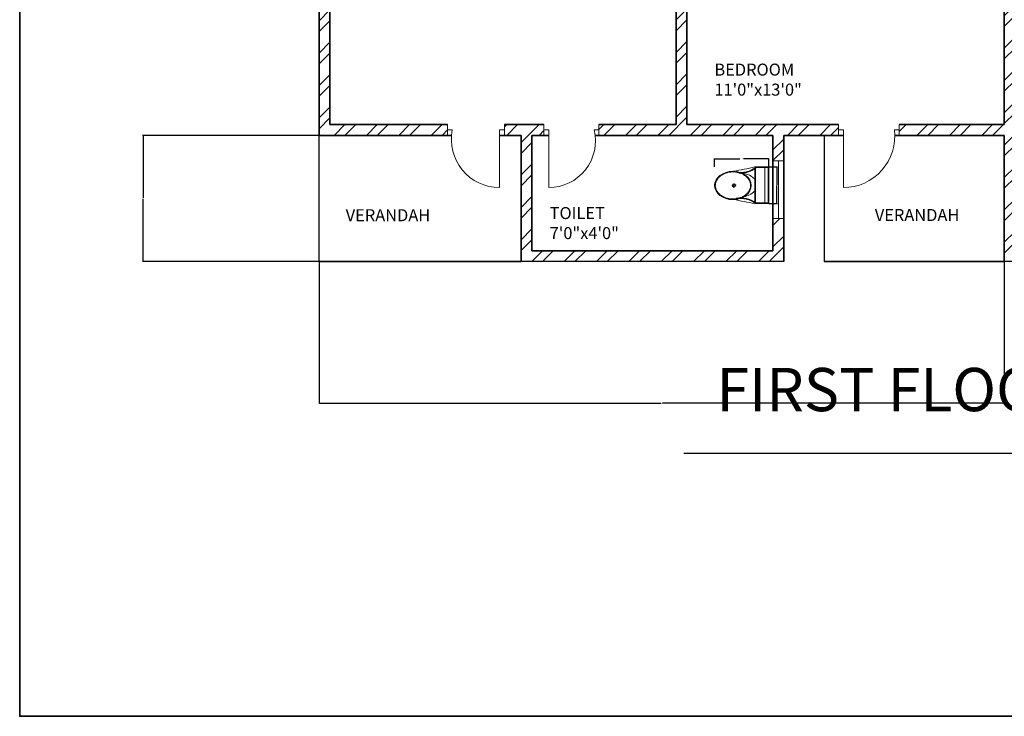
# Model space of a CAD drawing. Units: inches. Extents: x 1962 to 2771, y 1245 to 2660.
# Tile 1 of 114: x 1962 to 2371, y 1245 to 1534. Entities that reach past the tile are written whole.
import ezdxf

# ---------------------------------------------------------------- set-up
doc = ezdxf.new("R2010")
doc.units = ezdxf.units.IN
for name, color, linetype, lineweight in [('A-ANNO-DIMS', 2, 'Continuous', 18), ('A-ANNO-TEXT', 7, 'Continuous', 25), ('A-ANNO-TTLB', 7, 'Continuous', 35), ('A-AREA-IDEN', 7, 'Continuous', 18), ('A-DOOR', 3, 'Continuous', 18), ('A-FLOR-BALC', 7, 'Continuous', 25), ('A-FLOR-FIXT', 8, 'Continuous', 18), ('A-GLAZ', 4, 'Continuous', 18), ('A-WALL', 7, 'Continuous', 35), ('A-WALL-PATT', 252, 'Continuous', 13)]:
    doc.layers.add(name, color=color, linetype=linetype, lineweight=lineweight)
doc.styles.get("Standard").update_dxf_attribs({"font": 'arial.ttf'})
doc.dimstyles.get("Standard").update_dxf_attribs({"dimtxt": 0.18, "dimasz": 0.18, "dimexe": 0.18, "dimexo": 0.0625, "dimgap": 0.09, "dimtad": 0, "dimtih": 1, "dimtoh": 1, "dimdec": 4, "dimzin": 0, "dimdsep": 46, "dimtxsty": 'Standard', "dimcen": 0.09, "dimadec": 0, "dimazin": 0, "dimtfac": 1, "dimtdec": 4, "dimtofl": 0, "dimtmove": 0, "dimatfit": 3, "dimfxl": 1, "dimtolj": 1, "dimtzin": 0, "dimarcsym": 0})

# ---------------------------------------------------------------- blocks, each defined once
blk = doc.blocks.new('A$C31115884')
for p, q in [((283, 498), (223, 498)), ((258, 466), (258, 523)), ((0, 200), (0, 0)), ((520, 200), (0, 200)), ((10, 190), (10, 10)), ((510, 190), (10, 190)), ((510, 10), (510, 190)), ((520, 0), (520, 200)), ((510, 54), (0, 54)), ((10, 10), (510, 10)), ((0, 0), (520, 0))]:
    blk.add_line(p, q)
blk.add_circle((256, 496), 23.6)
for centre, radius, start, end in [((2778, -205), 2807, 165.4549, 171.7133), ((-295, 403), 365, 324.2091, 9.3499), ((-295, 403), 375, 324.2091, 9.3499), ((806, 403), 365, 170.6501, 215.7909), ((3237, 905), 2807, 188.2867, 194.5451), ((384, 406), 293, 190.2774, 224.1564), ((139, 406), 293, 315.8436, 2.6563), ((806, 403), 375, 179.2036, 215.7909)]:
    blk.add_arc(centre, radius, start, end)
blk.add_ellipse((256, 510), major_axis=(0, -261), ratio=0.772727)
blk.add_open_spline([(256, 259), (263, 259), (270, 260), (288, 262), (299, 265), (320, 273), (330, 278), (350, 291), (360, 299), (378, 316), (386, 326), (402, 347), (409, 358), (421, 383), (427, 395), (436, 422), (440, 436), (445, 465), (447, 480), (448, 509), (448, 524), (445, 553), (443, 568), (436, 596), (432, 610), (422, 636), (416, 649), (402, 672), (395, 683), (379, 703), (370, 712), (351, 728), (341, 735), (321, 746), (310, 751), (289, 757), (278, 759), (256, 761), (245, 761), (223, 757), (212, 754), (191, 746), (181, 741), (161, 728), (151, 720), (133, 703), (125, 693), (110, 672), (103, 660), (90, 636), (85, 623), (76, 596), (72, 582), (67, 553), (66, 538), (64, 509), (65, 494), (68, 465), (70, 450), (77, 422), (81, 408), (91, 382), (97, 370), (111, 346), (118, 335), (135, 316), (144, 307), (162, 291), (172, 284), (193, 273), (203, 269), (225, 262), (236, 260), (250, 259), (253, 259), (256, 259)], degree=3, knots=[0, 0, 0, 0, 0.110105, 0.110105, 0.285049, 0.285049, 0.459994, 0.459994, 0.634938, 0.634938, 0.809882, 0.809882, 0.984827, 0.984827, 1.159771, 1.159771, 1.334715, 1.334715, 1.50966, 1.50966, 1.684604, 1.684604, 1.859549, 1.859549, 2.034493, 2.034493, 2.209437, 2.209437, 2.384382, 2.384382, 2.559326, 2.559326, 2.73427, 2.73427, 2.909215, 2.909215, 3.084159, 3.084159, 3.259103, 3.259103, 3.434048, 3.434048, 3.608992, 3.608992, 3.783936, 3.783936, 3.958881, 3.958881, 4.133825, 4.133825, 4.30877, 4.30877, 4.483714, 4.483714, 4.658658, 4.658658, 4.833603, 4.833603, 5.008547, 5.008547, 5.183491, 5.183491, 5.358436, 5.358436, 5.53338, 5.53338, 5.708324, 5.708324, 5.883269, 5.883269, 6.058213, 6.058213, 6.233158, 6.233158, 6.283185, 6.283185, 6.283185, 6.283185])
blk = doc.blocks.new('WIN-24IN-A')
for p, q in [((0, 24), (4.5, 24)), ((4.5, 24), (2.25, 24)), ((2.25, 24), (2.25, 0)), ((2.25, 0), (0, 0)), ((0, 0), (4.5, 0))]:
    blk.add_line(p, q)
blk = doc.blocks.new('*D16')
at = {"layer": 'A-ANNO-DIMS', "color": 0, "lineweight": -2, "transparency": 16777216}
for p, q in [((2250.8, 1473.28), (2250.8, 1476.77)), ((2250.98, 1476.59), (2261.29, 1476.59)), ((2273.16, 1476.59), (2262.85, 1476.59)), ((2273.34, 1473.28), (2273.34, 1476.77))]:
    blk.add_line(p, q, dxfattribs=at)
at = {"layer": 'A-ANNO-DIMS', "color": 0, "transparency": 16777216}
for points in [[(2250.98, 1476.62), (2250.98, 1476.56), (2250.8, 1476.59)], [(2273.16, 1476.62), (2273.16, 1476.56), (2273.34, 1476.59)]]:
    blk.add_solid(points, dxfattribs=at)
at = {"layer": 'Defpoints', "color": 0, "transparency": 16777216}
for p in [(2250.8, 1476.59), (2250.8, 1473.21), (2273.34, 1473.21)]:
    blk.add_point(p, dxfattribs=at)
at = {"layer": 'A-ANNO-DIMS', "color": 0, "transparency": 16777216, "insert": (2262.07, 1476.59), "char_height": 0.18, "attachment_point": 5}
blk.add_mtext('\\A1;WC 23 TYP.', dxfattribs=at)
blk = doc.blocks.new('*D17')
at = {"layer": 'A-ANNO-DIMS', "color": 0, "lineweight": -2, "transparency": 16777216}
for p, q in [((2273.4, 1473.21), (2276.9, 1473.21)), ((2276.72, 1473.03), (2276.72, 1465.79)), ((2276.72, 1458.18), (2276.72, 1465.43)), ((2273.4, 1458), (2276.9, 1458))]:
    blk.add_line(p, q, dxfattribs=at)
at = {"layer": 'A-ANNO-DIMS', "color": 0, "transparency": 16777216}
for points in [[(2276.69, 1473.03), (2276.75, 1473.03), (2276.72, 1473.21)], [(2276.69, 1458.18), (2276.75, 1458.18), (2276.72, 1458)]]:
    blk.add_solid(points, dxfattribs=at)
at = {"layer": 'Defpoints', "color": 0, "transparency": 16777216}
for p in [(2273.34, 1473.21), (2276.72, 1473.21), (2273.34, 1458)]:
    blk.add_point(p, dxfattribs=at)
at = {"layer": 'A-ANNO-DIMS', "color": 0, "transparency": 16777216, "insert": (2276.72, 1465.61), "char_height": 0.18, "attachment_point": 5}
blk.add_mtext('\\A1;15 TYP.', dxfattribs=at)
blk = doc.blocks.new('*D46')
at = {"layer": 'A-ANNO-DIMS', "color": 0, "lineweight": -2, "transparency": 16777216}
for p, q in [((2086.31, 1433.78), (2086.31, 1374.71)), ((2371.31, 1433.78), (2371.31, 1374.71)), ((2086.49, 1374.89), (2228.52, 1374.89)), ((2371.13, 1374.89), (2229.1, 1374.89))]:
    blk.add_line(p, q, dxfattribs=at)
at = {"layer": 'A-ANNO-DIMS', "color": 0, "transparency": 16777216}
for points in [[(2086.49, 1374.92), (2086.49, 1374.86), (2086.31, 1374.89)], [(2371.13, 1374.92), (2371.13, 1374.86), (2371.31, 1374.89)]]:
    blk.add_solid(points, dxfattribs=at)
at = {"layer": 'Defpoints', "color": 0, "transparency": 16777216}
for p in [(2086.31, 1433.84), (2371.31, 1433.84), (2086.31, 1374.89)]:
    blk.add_point(p, dxfattribs=at)
at = {"layer": 'A-ANNO-DIMS', "color": 0, "transparency": 16777216, "insert": (2228.81, 1374.89), "char_height": 0.18, "attachment_point": 5}
blk.add_mtext('\\A1;285', dxfattribs=at)
blk = doc.blocks.new('*D47')
at = {"layer": 'A-ANNO-DIMS', "color": 0, "lineweight": -2, "transparency": 16777216}
for p, q in [((2086.24, 1486.34), (2012.89, 1486.34)), ((2013.07, 1486.16), (2013.07, 1460.28)), ((2013.07, 1434.02), (2013.07, 1459.91)), ((2086.24, 1433.84), (2012.89, 1433.84))]:
    blk.add_line(p, q, dxfattribs=at)
at = {"layer": 'A-ANNO-DIMS', "color": 0, "transparency": 16777216}
for points in [[(2013.04, 1486.16), (2013.1, 1486.16), (2013.07, 1486.34)], [(2013.04, 1434.02), (2013.1, 1434.02), (2013.07, 1433.84)]]:
    blk.add_solid(points, dxfattribs=at)
at = {"layer": 'Defpoints', "color": 0, "transparency": 16777216}
for p in [(2013.07, 1486.34), (2086.31, 1486.34), (2086.31, 1433.84)]:
    blk.add_point(p, dxfattribs=at)
at = {"layer": 'A-ANNO-DIMS', "color": 0, "transparency": 16777216, "insert": (2013.07, 1460.09), "char_height": 0.18, "attachment_point": 5}
blk.add_mtext('\\A1;52.5', dxfattribs=at)

msp = doc.modelspace()

# ---------------------------------------------------------------- hatches: boundary and pattern name
at = {"layer": 'A-WALL-PATT'}
h = msp.add_hatch(dxfattribs=at)
h.set_pattern_fill('ANSI32', color=256)
h.paths.add_polyline_path([(2090.8074, 2467.3437), (2141.6481, 2467.3437), (2141.6481, 2469.5937), (2141.6481, 2471.8437), (2086.3074, 2471.8437), (2086.3074, 2422.5333), (2090.8074, 2422.5333)])
h.paths.add_polyline_path([(2282.7664, 2471.8437), (2204.8982, 2471.8437), (2204.8982, 2467.3437), (2234.8074, 2467.3437), (2234.8074, 2311.3437), (2228.7492, 2311.3437), (2228.7492, 2306.8437), (2234.8074, 2306.8437), (2331.9227, 2306.8437), (2331.9227, 2309.0937), (2331.9227, 2311.3437), (2239.3074, 2311.3437), (2239.3074, 2467.3437), (2282.7664, 2467.3437), (2282.7664, 2469.5937)])
h.paths.add_polyline_path([(2471.4531, 2519.8437), (2552.011, 2519.8437), (2564.3996, 2519.8437), (2564.3996, 2511.1389), (2568.8996, 2511.1389), (2568.8996, 2524.3437), (2466.9531, 2524.3437), (2466.9531, 2471.8437), (2450.0749, 2471.8437), (2446.4672, 2471.8437), (2446.4672, 2467.3437), (2450.0749, 2467.3437), (2475.9988, 2467.3437), (2475.9988, 2469.5937), (2475.9988, 2471.8437), (2471.4531, 2471.8437)])
h.paths.add_polyline_path([(2575.2231, 2469.5937), (2575.2231, 2471.8437), (2568.8996, 2471.8437), (2568.8996, 2487.1389), (2564.3996, 2487.1389), (2564.3996, 2471.8437), (2556.511, 2471.8437), (2499.2904, 2471.8437), (2499.2904, 2467.3437), (2507.8074, 2467.3437), (2507.8074, 2311.3437), (2414.863, 2311.3437), (2414.863, 2306.8437), (2512.3074, 2306.8437), (2517.0114, 2306.8437), (2517.0114, 2309.0937), (2517.0114, 2311.3437), (2512.3074, 2311.3437), (2512.3074, 2467.3437), (2575.2231, 2467.3437)])
h.paths.add_polyline_path([(2660.8074, 2471.8437), (2600.9602, 2471.8437), (2600.9602, 2467.3437), (2656.3074, 2467.3437), (2656.3074, 2432.5704), (2660.8074, 2432.5704)])
h.paths.add_polyline_path([(2660.8074, 2372.5704), (2656.3074, 2372.5704), (2656.3074, 2311.3437), (2600.276, 2311.3437), (2600.276, 2309.0937), (2600.276, 2306.8437), (2656.3074, 2306.8437), (2656.3074, 2296.2593), (2660.8074, 2296.2593)])
h.paths.add_polyline_path([(2572.3074, 2306.8437), (2577.1385, 2306.8437), (2577.1385, 2311.3437), (2551.082, 2311.3437), (2551.082, 2306.8437), (2567.8074, 2306.8437), (2567.8074, 2258.8437), (2540.0574, 2258.8437), (2540.0574, 2256.5937), (2540.0574, 2254.3437), (2567.8074, 2254.3437), (2656.3074, 2254.3437), (2656.3074, 2236.9085), (2660.8074, 2236.9085), (2660.8074, 2272.2593), (2656.3074, 2272.2593), (2656.3074, 2258.8437), (2572.3074, 2258.8437)])
h.paths.add_polyline_path([(2512.3074, 2254.3437), (2518.8716, 2254.3437), (2518.8716, 2256.5937), (2518.8716, 2258.8437), (2507.8074, 2258.8437), (2507.8074, 2177.8437), (2567.8074, 2177.8437), (2567.8074, 2172.9628), (2572.3074, 2172.9628), (2572.3074, 2177.8437), (2656.3074, 2177.8437), (2656.3074, 2166.4846), (2660.8074, 2166.4846), (2660.8074, 2200.9085), (2656.3074, 2200.9085), (2656.3074, 2182.3437), (2512.3074, 2182.3437)])
h.paths.add_polyline_path([(2656.3074, 2129.8437), (2572.3074, 2129.8437), (2572.3074, 2150.3044), (2570.0574, 2150.3044), (2567.8074, 2150.3044), (2567.8074, 2129.8437), (2507.8074, 2129.8437), (2507.8074, 2116.3027), (2510.0574, 2116.3027), (2512.3074, 2116.3027), (2512.3074, 2125.3437), (2567.8074, 2125.3437), (2572.3074, 2125.3437), (2656.3074, 2125.3437)])
h.paths.add_polyline_path([(2090.8074, 2362.5333), (2086.3074, 2362.5333), (2086.3074, 2298.6242), (2090.8074, 2298.6242), (2090.8074, 2306.8437), (2174.8074, 2306.8437), (2174.8074, 2286.4178), (2179.3074, 2286.4178), (2179.3074, 2306.8437), (2192.8641, 2306.8437), (2192.8641, 2309.0937), (2192.8641, 2311.3437), (2090.8074, 2311.3437)])
h.paths.add_polyline_path([(2209.156, 2258.8437), (2179.3074, 2258.8437), (2179.3074, 2263.2236), (2177.0574, 2263.2236), (2174.8074, 2263.2236), (2174.8074, 2258.8437), (2090.8074, 2258.8437), (2090.8074, 2274.6242), (2086.3074, 2274.6242), (2086.3074, 2238.2967), (2088.5574, 2238.2967), (2090.8074, 2238.2967), (2090.8074, 2254.3437), (2209.156, 2254.3437)])
h.paths.add_polyline_path([(2090.8074, 2177.8437), (2234.8074, 2177.8437), (2234.8074, 2173.1428), (2239.3074, 2173.1428), (2239.3074, 2258.8437), (2230.8442, 2258.8437), (2230.8442, 2256.5937), (2230.8442, 2254.3437), (2234.8074, 2254.3437), (2234.8074, 2182.3437), (2090.8074, 2182.3437), (2090.8074, 2202.2967), (2086.3074, 2202.2967), (2086.3074, 2140.0389), (2090.8074, 2140.0389)])
h.paths.add_polyline_path([(2090.8074, 2080.0389), (2086.3074, 2080.0389), (2086.3074, 2033.8437), (2090.8074, 2033.8437)], flags=17)
h.paths.add_polyline_path([(2244.9405, 2033.8437), (2239.3074, 2033.8437), (2239.3074, 2142.0665), (2237.2592, 2142.0665), (2234.8074, 2142.0665), (2234.8074, 2033.8437), (2090.8074, 2033.8437), (2076.5204, 2033.8437), (2072.0204, 2033.8437), (2072.0204, 2000.4493), (2076.5204, 2000.4493), (2076.5204, 2029.3437), (2090.8074, 2029.3437), (2244.9405, 2029.3437), (2244.9405, 2031.5937)])
h.paths.add_polyline_path([(2234.8074, 1933.3437), (2076.5204, 1933.3437), (2076.5204, 1952.4493), (2074.2704, 1952.4493), (2072.0204, 1952.4493), (2072.0204, 1933.3437), (2072.0204, 1928.8437), (2234.8074, 1928.8437)])
h.paths.add_polyline_path([(2090.8074, 1928.8437), (2086.3074, 1928.8437), (2086.3074, 1906.5013), (2090.8074, 1906.5013)])
h.paths.add_polyline_path([(2090.8074, 1846.5013), (2086.3074, 1846.5013), (2086.3074, 1769.9917), (2088.5574, 1769.9917), (2090.8074, 1769.9917), (2090.8074, 1780.3437), (2234.8074, 1780.3437), (2234.8074, 1708.3437), (2230.3764, 1708.3437), (2230.3764, 1703.8437), (2239.3074, 1703.8437), (2239.3074, 1792.6669), (2237.0574, 1792.6669), (2234.8074, 1792.6669), (2234.8074, 1784.8437), (2090.8074, 1784.8437)])
h.paths.add_polyline_path([(2239.3074, 1928.8437), (2244.9405, 1928.8437), (2244.9405, 1931.0937), (2244.9405, 1933.3437), (2234.8074, 1933.3437), (2234.8074, 1928.8437), (2234.8074, 1825.5949), (2239.3074, 1825.5949)])
h.paths.add_polyline_path([(2148.0425, 1649.0937), (2148.0425, 1651.3437), (2090.8074, 1651.3437), (2090.8074, 1646.8437), (2148.0425, 1646.8437)], flags=0)
h.paths.add_polyline_path([(2207.5601, 1708.3437), (2090.8074, 1708.3437), (2090.8074, 1703.8437), (2174.8074, 1703.8437), (2174.8074, 1651.3437), (2170.4457, 1651.3437), (2170.4457, 1646.8437), (2195.9924, 1646.8437), (2195.9924, 1649.0937), (2195.9924, 1651.3437), (2179.3074, 1651.3437), (2179.3074, 1703.8437), (2207.5601, 1703.8437), (2207.5601, 1706.0937)])
h.paths.add_polyline_path([(2090.8074, 1733.9917), (2086.3074, 1733.9917), (2086.3074, 1696.1032), (2088.5574, 1696.1032), (2090.8074, 1696.1032)])
h.paths.add_polyline_path([(2090.8074, 1672.1032), (2086.3074, 1672.1032), (2086.3074, 1600.3335), (2090.8074, 1600.3335)])
h.paths.add_polyline_path([(2090.8074, 1540.3335), (2086.3074, 1540.3335), (2086.3074, 1486.3437), (2139.6766, 1486.3437), (2139.6766, 1490.8437), (2090.8074, 1490.8437)])
h.paths.add_polyline_path([(2302.3876, 1490.8437), (2239.3074, 1490.8437), (2239.3074, 1646.8437), (2335.9994, 1646.8437), (2335.9994, 1651.3437), (2229.884, 1651.3437), (2229.884, 1646.8437), (2234.8074, 1646.8437), (2234.8074, 1490.8437), (2202.7103, 1490.8437), (2202.7103, 1488.5937), (2202.7103, 1486.3437), (2275.0699, 1486.3437), (2275.0699, 1475.772), (2279.5699, 1475.772), (2279.5699, 1486.3437), (2302.3876, 1486.3437)])
h.paths.add_polyline_path([(2279.5699, 1451.772), (2275.0699, 1451.772), (2275.0699, 1438.3437), (2174.8074, 1438.3437), (2174.8074, 1486.3437), (2179.7922, 1486.3437), (2179.7922, 1490.8437), (2163.3585, 1490.8437), (2163.3585, 1488.5937), (2163.3585, 1486.3437), (2170.3074, 1486.3437), (2170.3074, 1433.8437), (2279.5699, 1433.8437)])
h.paths.add_polyline_path([(2427.2363, 1490.8437), (2375.8074, 1490.8437), (2375.8074, 1646.8437), (2381.6401, 1646.8437), (2381.6401, 1651.3437), (2365.887, 1651.3437), (2365.887, 1649.0937), (2365.887, 1646.8437), (2371.3074, 1646.8437), (2371.3074, 1490.8437), (2327.5627, 1490.8437), (2327.5627, 1488.5937), (2327.5627, 1486.3437), (2371.3074, 1486.3437), (2371.3074, 1433.8437), (2375.8074, 1433.8437), (2375.8074, 1486.3437), (2427.2363, 1486.3437)])
h.paths.add_polyline_path([(2512.3074, 1646.8437), (2519.4351, 1646.8437), (2519.4351, 1649.0937), (2519.4351, 1651.3437), (2507.8074, 1651.3437), (2416.0063, 1651.3437), (2416.0063, 1649.0937), (2416.0063, 1646.8437), (2507.8074, 1646.8437), (2507.8074, 1490.8437), (2497.0532, 1490.8437), (2497.0532, 1488.5937), (2497.0532, 1486.3437), (2574.9344, 1486.3437), (2574.9344, 1476.0181), (2579.4344, 1476.0181), (2579.4344, 1486.3437), (2584.4872, 1486.3437), (2584.3074, 1490.8437), (2512.3074, 1490.8437)])
h.paths.add_polyline_path([(2470.5091, 1486.3437), (2473.9767, 1486.3437), (2473.9767, 1490.8437), (2449.6605, 1490.8437), (2449.6605, 1488.5937), (2449.6605, 1486.3437), (2466.0091, 1486.3437), (2466.0091, 1433.8437), (2470.5091, 1433.8437), (2579.4344, 1433.8437), (2579.4344, 1452.0181), (2574.9344, 1452.0181), (2574.9344, 1438.3437), (2554.5091, 1438.3437), (2470.5091, 1438.3437)])
h.paths.add_polyline_path([(2656.3074, 1490.8437), (2611.86, 1490.8437), (2611.86, 1486.3437), (2656.3074, 1486.3437)])
h.paths.add_polyline_path([(2660.8074, 1532.7007), (2658.5574, 1532.7007), (2656.3074, 1532.7007), (2656.3074, 1486.3437), (2660.8074, 1486.3437)])
h.paths.add_polyline_path([(2660.8074, 1664.9663), (2656.3074, 1664.9663), (2656.3074, 1651.3437), (2602.2313, 1651.3437), (2602.2313, 1646.8437), (2656.3074, 1646.8437), (2656.3074, 1592.7007), (2660.8074, 1592.7007)])
h.paths.add_polyline_path([(2660.8074, 1724.5221), (2656.3074, 1724.5221), (2656.3074, 1703.8437), (2542.4725, 1703.8437), (2542.4725, 1699.3437), (2567.8074, 1699.3437), (2567.8074, 1651.3437), (2552.7766, 1651.3437), (2552.7766, 1649.0937), (2552.7766, 1646.8437), (2577.2878, 1646.8437), (2577.2878, 1649.0937), (2577.2878, 1651.3437), (2572.3074, 1651.3437), (2572.3074, 1699.3437), (2656.3074, 1699.3437), (2656.3074, 1688.9663), (2660.8074, 1688.9663)])
h.paths.add_polyline_path([(2660.8074, 1880.6524), (2656.3074, 1880.6524), (2656.3074, 1832.8437), (2512.3074, 1832.8437), (2512.3074, 1837.8959), (2507.8074, 1837.8959), (2507.8074, 1828.3437), (2567.8074, 1828.3437), (2567.8074, 1804.3437), (2572.3074, 1804.3437), (2572.3074, 1828.3437), (2656.3074, 1828.3437), (2656.3074, 1818.6778), (2660.8074, 1818.6778)])
h.paths.add_polyline_path([(2660.8074, 1794.6778), (2656.3074, 1794.6778), (2656.3074, 1780.3437), (2572.3074, 1780.3437), (2572.3074, 1783.0303), (2570.0574, 1783.0303), (2567.8074, 1783.0303), (2567.8074, 1780.3437), (2507.8074, 1780.3437), (2507.8074, 1699.3437), (2517.8858, 1699.3437), (2517.8858, 1701.5937), (2517.8858, 1703.8437), (2512.3074, 1703.8437), (2512.3074, 1775.8437), (2656.3074, 1775.8437), (2656.3074, 1760.5221), (2660.8074, 1760.5221)])
h.paths.add_polyline_path([(2660.8074, 1981.3437), (2660.8074, 2020.2808), (2658.5574, 2020.2808), (2656.3074, 2020.2808), (2656.3074, 1981.3437), (2512.3074, 1981.3437), (2512.3074, 2086.6996), (2507.8074, 2086.6996), (2507.8074, 1981.3437), (2375.8074, 1981.3437), (2375.8074, 1986.8505), (2373.5574, 1986.8505), (2371.3074, 1986.8505), (2371.3074, 1973.2607), (2375.8074, 1973.2607), (2375.8074, 1976.8437), (2507.8074, 1976.8437), (2507.8074, 1865.4281), (2510.0574, 1865.4281), (2512.3074, 1865.4281), (2512.3074, 1976.8437), (2660.8074, 1976.8437)])
h.paths.add_polyline_path([(2375.8074, 1940.297), (2373.5574, 1940.297), (2371.3074, 1940.297), (2371.3074, 1933.3437), (2278.4434, 1933.3437), (2278.4434, 1928.8437), (2371.3074, 1928.8437), (2371.3074, 1651.3437), (2375.8074, 1651.3437)])
h.paths.add_polyline_path([(2660.8074, 1976.8437), (2656.3074, 1976.8437), (2656.3074, 1940.6524), (2660.8074, 1940.6524)], flags=17)
h.paths.add_polyline_path([(2660.8074, 2142.4846), (2656.3074, 2142.4846), (2656.3074, 2080.2808), (2660.8074, 2080.2808)])
h.paths.add_polyline_path([(2381.4189, 2311.3437), (2375.8074, 2311.3437), (2375.8074, 2467.3437), (2424.7242, 2467.3437), (2424.7242, 2469.5937), (2424.7242, 2471.8437), (2375.8074, 2471.8437), (2375.8074, 2524.3437), (2371.3074, 2524.3437), (2371.3074, 2471.8437), (2307.2097, 2471.8437), (2307.2097, 2467.3437), (2371.3074, 2467.3437), (2371.3074, 2311.3437), (2366.8901, 2311.3437), (2366.8901, 2306.8437), (2371.3074, 2306.8437), (2371.3074, 2033.8437), (2279.6589, 2033.8437), (2279.6589, 2029.3437), (2371.3074, 2029.3437), (2371.3074, 2014.2598), (2375.8074, 2014.2598), (2375.8074, 2306.8437), (2381.4189, 2306.8437)])
h.paths.add_polyline_path([(2263.3074, 2524.3437), (2170.3074, 2524.3437), (2170.3074, 2519.8437), (2170.3074, 2471.8437), (2165.0312, 2471.8437), (2165.0312, 2467.3437), (2179.6721, 2467.3437), (2179.6721, 2469.5161), (2179.6721, 2471.8437), (2174.8074, 2471.8437), (2174.8074, 2519.8437), (2258.8074, 2519.8437), (2258.8074, 2511.6436), (2263.3074, 2511.6436)])
h.paths.add_polyline_path([(2245.0232, 1361.4123), (2492.9468, 1361.4123), (2492.9468, 1398.505), (2245.0232, 1398.505)], flags=9)
h.paths.add_polyline_path([(2388.1434, 2086.6936), (2425.0704, 2086.6936), (2425.0704, 2105.3509), (2388.1434, 2105.3509)], flags=9)
h.paths.add_polyline_path([(2404.922, 2242.6744), (2445.7337, 2242.6744), (2445.7337, 2261.3318), (2404.922, 2261.3318)], flags=9)
h.paths.add_polyline_path([(2269.4107, 2156.7935), (2306.3378, 2156.7935), (2306.3378, 2175.4508), (2269.4107, 2175.4508)], flags=9)
h.paths.add_polyline_path([(2269.3277, 2233.4343), (2306.2547, 2233.4343), (2306.2547, 2252.0917), (2269.3277, 2252.0917)], flags=9)
h.paths.add_polyline_path([(2431.6052, 2320.6922), (2470.4456, 2320.6922), (2470.4456, 2339.3495), (2431.6052, 2339.3495)], flags=25)
h.paths.add_polyline_path([(2249.6902, 2315.7608), (2288.5306, 2315.7608), (2288.5306, 2334.4182), (2249.6902, 2334.4182)], flags=25)
h.paths.add_polyline_path([(2096.9301, 2314.3181), (2135.7704, 2314.3181), (2135.7704, 2332.9755), (2096.9301, 2332.9755)], flags=25)
h.paths.add_polyline_path([(2134.3475, 2285.7089), (2161.4655, 2285.7089), (2161.4655, 2304.3662), (2134.3475, 2304.3662)], flags=9)
h.paths.add_polyline_path([(2126.5155, 2209.4076), (2159.9227, 2209.4076), (2159.9227, 2228.065), (2126.5155, 2228.065)], flags=25)
h.paths.add_polyline_path([(2110.5753, 2141.5299), (2149.4157, 2141.5299), (2149.4157, 2160.1872), (2110.5753, 2160.1872)], flags=25)
h.paths.add_polyline_path([(2249.8618, 1968.3317), (2286.3966, 1968.3317), (2286.3966, 1986.989), (2249.8618, 1986.989)], flags=9)
h.paths.add_polyline_path([(2395.9507, 1777.0051), (2436.7624, 1777.0051), (2436.7624, 1795.6625), (2395.9507, 1795.6625)], flags=9)
h.paths.add_polyline_path([(2398.5259, 1888.5651), (2435.0062, 1888.5651), (2435.0062, 1907.2224), (2398.5259, 1907.2224)], flags=25)
h.paths.add_polyline_path([(2259.3506, 1728.3559), (2296.2776, 1728.3559), (2296.2776, 1747.0132), (2259.3506, 1747.0132)], flags=9)
h.paths.add_polyline_path([(2271.3698, 1845.268), (2308.2968, 1845.268), (2308.2968, 1863.9253), (2271.3698, 1863.9253)], flags=9)
h.paths.add_polyline_path([(2120.9355, 1786.3027), (2159.7759, 1786.3027), (2159.7759, 1804.9601), (2120.9355, 1804.9601)], flags=25)
h.paths.add_polyline_path([(2121.3164, 1732.1043), (2154.7236, 1732.1043), (2154.7236, 1750.7616), (2121.3164, 1750.7616)], flags=25)
h.paths.add_polyline_path([(2118.3706, 1678.8997), (2147.5282, 1678.8997), (2147.5282, 1697.557), (2118.3706, 1697.557)], flags=25)
h.paths.add_polyline_path([(2385.9227, 1493.557), (2424.763, 1493.557), (2424.763, 1512.2143), (2385.9227, 1512.2143)], flags=25)
h.paths.add_polyline_path([(2248.7058, 1500.0256), (2287.5462, 1500.0256), (2287.5462, 1518.6829), (2248.7058, 1518.6829)], flags=25)
h.paths.add_polyline_path([(2104.1669, 1617.3771), (2143.0073, 1617.3771), (2143.0073, 1636.0344), (2104.1669, 1636.0344)], flags=9)
h.paths.add_polyline_path([(2096.0714, 1447.8824), (2137.3845, 1447.8824), (2137.3845, 1458.1859), (2096.0714, 1458.1859)], flags=9)
h.paths.add_polyline_path([(2180.6114, 1440.325), (2209.7689, 1440.325), (2209.7689, 1458.9823), (2180.6114, 1458.9823)], flags=25)
h.paths.add_polyline_path([(2316.1698, 1447.9637), (2357.4829, 1447.9637), (2357.4829, 1458.2673), (2316.1698, 1458.2673)], flags=9)
h.paths.add_polyline_path([(2397.6187, 1447.9637), (2438.9318, 1447.9637), (2438.9318, 1458.2673), (2397.6187, 1458.2673)], flags=9)
h.paths.add_polyline_path([(2473.0778, 1439.5953), (2502.2354, 1439.5953), (2502.2354, 1458.2527), (2473.0778, 1458.2527)], flags=25)
h.paths.add_polyline_path([(2589.7027, 1447.8819), (2631.0158, 1447.8819), (2631.0158, 1458.1855), (2589.7027, 1458.1855)], flags=9)
h.paths.add_polyline_path([(2522.4009, 1497.5285), (2561.2413, 1497.5285), (2561.2413, 1516.1859), (2522.4009, 1516.1859)], flags=25)
h.paths.add_polyline_path([(2579.6565, 1671.3482), (2608.8141, 1671.3482), (2608.8141, 1690.0056), (2579.6565, 1690.0056)], flags=25)
h.paths.add_polyline_path([(2544.7038, 1725.5064), (2578.1111, 1725.5064), (2578.1111, 1744.1637), (2544.7038, 1744.1637)], flags=25)
h.paths.add_polyline_path([(2578.1191, 1807.472), (2607.2766, 1807.472), (2607.2766, 1826.1293), (2578.1191, 1826.1293)], flags=25)
h.paths.add_polyline_path([(2595.0614, 1835.1839), (2633.9018, 1835.1839), (2633.9018, 1853.8413), (2595.0614, 1853.8413)], flags=25)
h.paths.add_polyline_path([(2567.0097, 2097.7035), (2605.8501, 2097.7035), (2605.8501, 2116.3609), (2567.0097, 2116.3609)], flags=9)
h.paths.add_polyline_path([(2586.644, 2134.6454), (2615.8015, 2134.6454), (2615.8015, 2153.3027), (2586.644, 2153.3027)], flags=9)
h.paths.add_polyline_path([(2544.6185, 2212.6783), (2578.0258, 2212.6783), (2578.0258, 2231.3356), (2544.6185, 2231.3356)], flags=25)
h.paths.add_polyline_path([(2577.0273, 2256.9023), (2606.1849, 2256.9023), (2606.1849, 2275.5597), (2577.0273, 2275.5597)], flags=24)
h.paths.add_polyline_path([(2605.2683, 2315.2821), (2644.1087, 2315.2821), (2644.1087, 2333.9395), (2605.2683, 2333.9395)], flags=25)
h.paths.add_polyline_path([(2583.1244, 2496.1815), (2624.4375, 2496.1815), (2624.4375, 2506.4851), (2583.1244, 2506.4851)], flags=9)
h.paths.add_polyline_path([(2474.761, 2497.0823), (2503.9185, 2497.0823), (2503.9185, 2515.7397), (2474.761, 2515.7397)], flags=25)
h.paths.add_polyline_path([(2387.5787, 2494.2563), (2428.902, 2494.2563), (2428.902, 2504.5598), (2387.5787, 2504.5598)], flags=9)
h.paths.add_polyline_path([(2300.1657, 2500.1564), (2341.4788, 2500.1564), (2341.4788, 2510.46), (2300.1657, 2510.46)], flags=25)
h.paths.add_polyline_path([(2176.8589, 2497.5843), (2206.0165, 2497.5843), (2206.0165, 2516.2416), (2176.8589, 2516.2416)], flags=25)
h.paths.add_polyline_path([(2097.4668, 2494.9762), (2138.7799, 2494.9762), (2138.7799, 2505.2798), (2097.4668, 2505.2798)], flags=9)

# ---------------------------------------------------------------- linework, layer by layer
at = {"layer": 'A-ANNO-TEXT'}
msp.add_line((2237.9561, 1354.1083), (2502.9067, 1354.1083), dxfattribs=at)
at = {"layer": 'A-ANNO-TTLB'}
msp.add_lwpolyline([(1961.7365, 2660.2579), (2771.213, 2660.2579), (2771.213, 1244.5817), (1961.7365, 1244.5817)], close=True, dxfattribs=at)
at = {"layer": 'A-DOOR'}
for p, q in [((2139.6766, 1486.3437), (2139.6766, 1490.8437)), ((2139.6766, 1490.8437), (2139.6766, 1488.5937)), ((2163.3585, 1486.3437), (2163.3585, 1490.8437)), ((2163.3585, 1490.8437), (2163.3585, 1488.5937)), ((2179.7922, 1486.3437), (2179.7922, 1490.8437)), ((2179.7922, 1490.8437), (2179.7922, 1488.5937)), ((2202.7103, 1486.3437), (2202.7103, 1490.8437)), ((2202.7103, 1490.8437), (2202.7103, 1488.5937)), ((2302.3876, 1486.3437), (2302.3876, 1490.8437)), ((2302.3876, 1490.8437), (2302.3876, 1488.5937)), ((2327.5627, 1486.3437), (2327.5627, 1490.8437)), ((2327.5627, 1490.8437), (2327.5627, 1488.5937)), ((2139.6766, 1488.5937), (2141.6766, 1488.5937)), ((2163.3585, 1488.5937), (2161.3585, 1488.5937)), ((2161.3585, 1488.5937), (2161.3585, 1464.5937)), ((2179.7922, 1488.5937), (2181.7922, 1488.5937)), ((2181.7922, 1488.5937), (2181.7922, 1464.5937)), ((2202.7103, 1488.5937), (2200.7103, 1488.5937)), ((2302.3876, 1488.5937), (2304.3876, 1488.5937)), ((2304.3876, 1488.5937), (2304.3876, 1464.5937)), ((2327.5627, 1488.5937), (2325.5627, 1488.5937))]:
    msp.add_line(p, q, dxfattribs=at)
for centre, radius, start, end in [((2161.3585, 1484.6641), 20.0704, 168.709048, 270), ((2181.7922, 1484.0498), 19.4561, 270, 13.50582), ((2304.3876, 1485.9351), 21.3414, 270, 7.156293)]:
    msp.add_arc(centre, radius, start, end, dxfattribs=at)
at = {"layer": 'A-FLOR-BALC'}
for p, q in [((2086.3074, 1433.8437), (2086.3074, 1486.3437)), ((2296.3835, 1486.3437), (2296.3835, 1433.8437)), ((2086.3074, 1433.8437), (2170.3074, 1433.8437)), ((2279.5699, 1433.8437), (2086.3074, 1433.8437)), ((2296.3835, 1433.8437), (2371.3074, 1433.8437)), ((2454.9439, 1433.8437), (2296.3835, 1433.8437))]:
    msp.add_line(p, q, dxfattribs=at)
at = {"layer": 'A-WALL'}
for p, q in [((2086.3074, 1928.8437), (2086.3074, 1486.3437)), ((2090.8074, 1780.3437), (2090.8074, 1490.8437)), ((2234.8074, 1646.8437), (2234.8074, 1490.8437)), ((2239.3074, 1646.8437), (2239.3074, 1490.8437)), ((2371.3074, 1646.8437), (2371.3074, 1490.8437)), ((2139.6766, 1490.8437), (2090.8074, 1490.8437)), ((2179.7922, 1490.8437), (2163.3585, 1490.8437)), ((2170.3074, 1490.8437), (2174.8074, 1490.8437)), ((2234.8074, 1490.8437), (2202.7103, 1490.8437)), ((2302.3876, 1490.8437), (2239.3074, 1490.8437)), ((2258.8074, 1490.8437), (2263.3074, 1490.8437)), ((2371.3074, 1490.8437), (2327.5627, 1490.8437)), ((2141.3585, 1486.3437), (2086.3074, 1486.3437)), ((2170.3074, 1486.3437), (2161.3585, 1486.3437)), ((2170.3074, 1433.8437), (2170.3074, 1486.3437)), ((2174.8074, 1486.3437), (2174.8074, 1438.3437)), ((2181.7922, 1486.3437), (2174.8074, 1486.3437)), ((2275.0699, 1486.3437), (2201.1126, 1486.3437)), ((2275.0699, 1438.3437), (2275.0699, 1486.3437)), ((2279.5699, 1486.3437), (2279.5699, 1433.8437)), ((2304.3876, 1486.3437), (2279.5699, 1486.3437)), ((2371.3074, 1486.3437), (2325.725, 1486.3437)), ((2371.3074, 1433.8437), (2371.3074, 1486.3437)), ((2174.8074, 1438.3437), (2275.0699, 1438.3437))]:
    msp.add_line(p, q, dxfattribs=at)

# ---------------------------------------------------------------- block references
at = {"layer": 'A-FLOR-FIXT', "xscale": 0.0292470664339069, "yscale": 0.0292470664339069, "zscale": 0.0292470664339069, "rotation": 89.99999999999999}
msp.add_blockref('A$C31115884', (2273.3373, 1458.0043), dxfattribs=at)
at = {"layer": 'A-GLAZ'}
msp.add_blockref('WIN-24IN-A', (2275.0699, 1451.772), dxfattribs=at)

# ---------------------------------------------------------------- texts
at = {"layer": 'A-ANNO-TEXT', "insert": (2251.5859, 1389.5603), "char_height": 18, "attachment_point": 1}
msp.add_mtext_dynamic_manual_height_columns('FIRST FLOOR PLAN', width=968.531758, gutter_width=12.5, heights=[0], dxfattribs=at)
at = {"layer": 'A-AREA-IDEN', "char_height": 5, "attachment_point": 1}
for s, width, insert in [('BEDROOM\\P11\'0"x13\'0"', 129.183964, (2250.7164, 1516.1983)), ('VERANDAH', 116.073154, (2097.3521, 1455.6126)), ('TOILET\\P7\'0"x4\'0"', 106.178658, (2182.1922, 1456.4977)), ('VERANDAH', 111.515445, (2317.4505, 1455.6939))]:
    msp.add_mtext_dynamic_manual_height_columns(s, width=width, gutter_width=12.5, heights=[0], dxfattribs=dict(at, insert=insert))

# ---------------------------------------------------------------- dimensions: what is measured, and where the dimension line sits
at = {"layer": 'A-ANNO-DIMS'}
for base, p1, p2, angle, override, picture, middle in [((2013.0704, 1486.3437), (2086.3074, 1433.8437), (2086.3074, 1486.3437), 90, {"dimdec": 1, "dimlfac": 1, "dimrnd": 0, "dimzin": 0, "dimdsep": 46, "dimlunit": 2}, '*D47', (2013.0704, 1460.0937)), ((2086.3074, 1374.8937), (2371.3074, 1433.8437), (2086.3074, 1433.8437), 180, {"dimdec": 0, "dimlfac": 1, "dimrnd": 0, "dimzin": 0, "dimdsep": 46, "dimlunit": 2}, '*D46', (2228.8074, 1374.8937))]:
    dim = msp.add_linear_dim(base=base, p1=p1, p2=p2, angle=angle, dimstyle='Standard', override=override, dxfattribs=at)
    dim.commit()
    dim.dimension.update_dxf_attribs({"geometry": picture, "text_midpoint": middle})
for base, p1, p2, angle, text, picture, middle in [((2250.8004, 1476.5933), (2273.3373, 1473.2128), (2250.8004, 1473.2128), 180, 'WC <> TYP.', '*D16', (2262.0689, 1476.5933)), ((2276.7179, 1473.2128), (2273.3373, 1458.0043), (2273.3373, 1473.2128), 90, '<> TYP.', '*D17', (2276.7179, 1465.6085))]:
    dim = msp.add_linear_dim(base=base, p1=p1, p2=p2, angle=angle, text=text, dimstyle='Standard', override={"dimdec": 0, "dimlfac": 1, "dimrnd": 0, "dimzin": 0, "dimdsep": 46, "dimlunit": 2}, dxfattribs=at)
    dim.commit()
    dim.dimension.update_dxf_attribs({"geometry": picture, "text_midpoint": middle})

doc.saveas('drawing.dxf')
